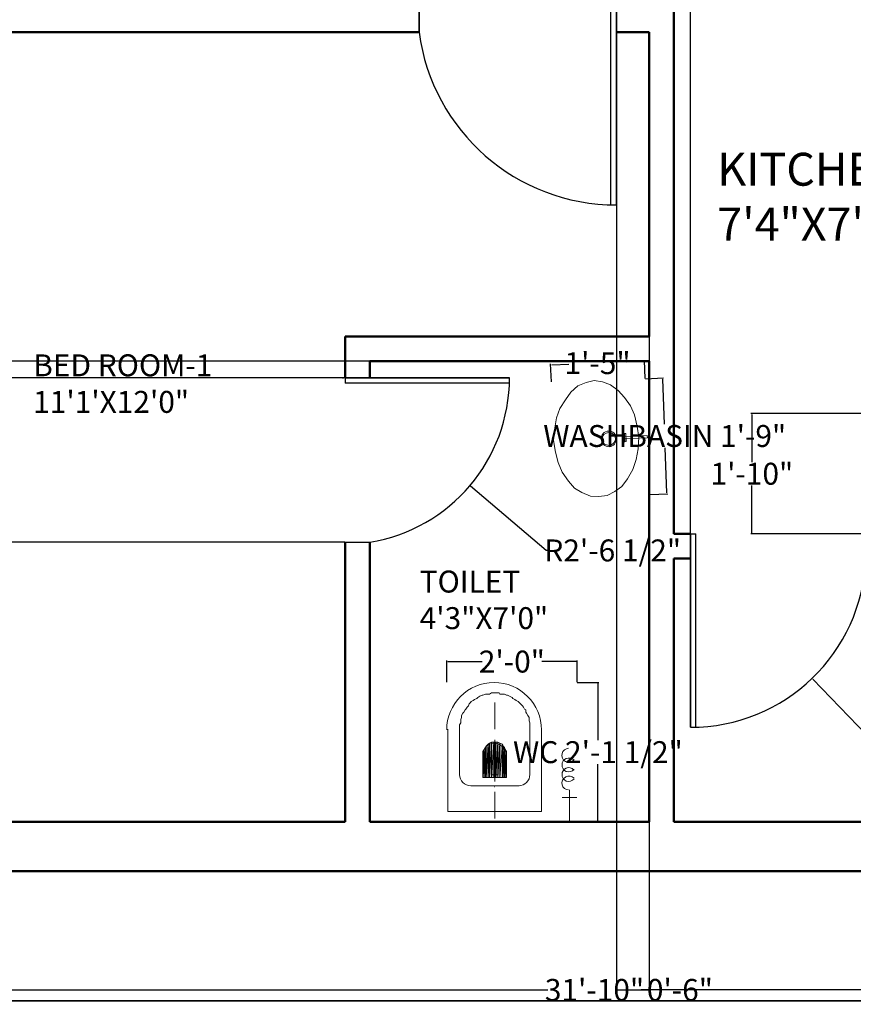
# Model space of a CAD drawing. Units: inches. Extents: x 124 to 591, y 365 to 713.
# Tile 2 of 5: x 266 to 418, y 365 to 545. Entities that reach past the tile are written whole.
import ezdxf

# ---------------------------------------------------------------- set-up
doc = ezdxf.new("R2010")
doc.units = ezdxf.units.IN
doc.header["$MEASUREMENT"] = 0
for name, color, linetype, lineweight in [('A-ANNO-DIMS', 2, 'Continuous', 18), ('A-ANNO-TTLB', 7, 'Continuous', 35), ('A-AREA-IDEN', 7, 'Continuous', 25), ('A-DOOR', 4, 'Continuous', 25), ('A-FLOR-FIXT', 8, 'Continuous', 18), ('A-WALL', 7, 'Continuous', 50)]:
    doc.layers.add(name, color=color, linetype=linetype, lineweight=lineweight)
doc.styles.get("Standard").update_dxf_attribs({"font": 'arial.ttf'})
doc.dimstyles.get("Standard").update_dxf_attribs({"dimtxt": 4, "dimasz": 0.18, "dimexe": 0.18, "dimexo": 0.0625, "dimgap": 0.09, "dimtad": 0, "dimtih": 1, "dimtoh": 1, "dimdec": 1, "dimzin": 0, "dimdsep": 46, "dimlunit": 3, "dimtxsty": 'Standard', "dimcen": 0.09, "dimclrd": 6, "dimclrt": 3, "dimadec": 0, "dimazin": 0, "dimtfac": 1, "dimtdec": 1, "dimtofl": 0, "dimtmove": 0, "dimatfit": 3, "dimfxl": 1, "dimtfillclr": 6, "dimtolj": 1, "dimtzin": 0, "dimarcsym": 0})

# ---------------------------------------------------------------- blocks, each defined once
blk = doc.blocks.new('WASH')
for p, q in [((268674.25, -2306.86), (268674.25, -2306.65)), ((268674.71, -2306.29), (268675.07, -2306.29)), ((268675.53, -2306.86), (268675.53, -2306.65)), ((268674.71, -2310.15), (268675.07, -2310.15))]:
    blk.add_line(p, q)
for points in [[(268665.93, -2302.29), (268666.07, -2301.01), (268666.64, -2299.72), (268667.36, -2298.58), (268668.5, -2297.72), (268669.93, -2296.79), (268671.43, -2296.22), (268673.07, -2295.86), (268674.86, -2295.65), (268676.5, -2295.86), (268678.36, -2296.22), (268679.78, -2296.79), (268681.07, -2297.72), (268682.21, -2298.58), (268683.14, -2299.72), (268683.64, -2301.01), (268683.86, -2302.29), (268683.64, -2303.58), (268683.14, -2304.79), (268682.21, -2305.94), (268681.07, -2306.86), (268679.78, -2307.72), (268678.36, -2308.29), (268676.5, -2308.65), (268674.86, -2308.86), (268673.07, -2308.65), (268671.43, -2308.29), (268669.93, -2307.72), (268668.5, -2306.86), (268667.36, -2305.94), (268666.64, -2304.79), (268666.07, -2303.58)], [(268674.14, -2306.65), (268674.14, -2306.65)], [(268674.86, -2306.29), (268674.86, -2306.29)], [(268675.43, -2306.65), (268675.43, -2306.65)]]:
    blk.add_lwpolyline(points, close=True)
for points in [[(268674.25, -2306.65), (268675.53, -2306.65), (268675.53, -2306.65)], [(268674.25, -2306.86), (268675.53, -2306.86), (268675.53, -2306.86)], [(268674.71, -2310.15), (268674.71, -2306.29), (268674.71, -2306.29)], [(268675.07, -2310.15), (268675.07, -2306.29), (268675.07, -2306.29)]]:
    blk.add_lwpolyline(points)
for points in [[(268673.57, -2304.22), (268673.57, -2304.86), (268674.14, -2305.36), (268674.78, -2305.36), (268674.78, -2305.36), (268675.43, -2305.36), (268676, -2304.86), (268676, -2304.22), (268676, -2304.22), (268676, -2303.51), (268675.43, -2303.01), (268674.78, -2303.01), (268674.78, -2303.01), (268674.14, -2303.01), (268673.57, -2303.51), (268673.57, -2304.22)], [(268673.78, -2304.22), (268673.78, -2304.72), (268674.21, -2305.22), (268674.78, -2305.22), (268674.78, -2305.22), (268675.36, -2305.22), (268675.78, -2304.72), (268675.78, -2304.22), (268675.78, -2304.22), (268675.78, -2303.65), (268675.36, -2303.15), (268674.78, -2303.15), (268674.78, -2303.15), (268674.21, -2303.15), (268673.78, -2303.65), (268673.78, -2304.22)]]:
    blk.add_open_spline(points, degree=3, knots=[0, 0, 0, 0, 0.0625, 0.0625, 0.0625, 0.062501, 0.125, 0.125, 0.125, 0.125001, 0.1875, 0.1875, 0.1875, 0.187501, 1, 1, 1, 1])
blk = doc.blocks.new('I')
h = blk.add_hatch(color=256)
h.paths.add_polyline_path([(268653.64, -2262.22), (268658.43, -2262.22), (268653.64, -2262.01)])
h.paths.add_polyline_path([(268658.43, -2262.22), (268653.64, -2262.01), (268658.07, -2262.01)])
h.paths.add_polyline_path([(268653.64, -2262.01), (268658.07, -2262.01), (268657.71, -2262.01)])
h = blk.add_hatch(color=256)
h.paths.add_polyline_path([(268653.64, -2262.44), (268658.78, -2262.44), (268653.64, -2262.22)])
h.paths.add_polyline_path([(268658.78, -2262.44), (268653.64, -2262.22), (268658.43, -2262.22)])
h = blk.add_hatch(color=256)
h.paths.add_polyline_path([(268653.64, -2262.58), (268659, -2262.58), (268653.64, -2262.44)])
h.paths.add_polyline_path([(268659, -2262.58), (268653.64, -2262.44), (268658.78, -2262.44)])
h = blk.add_hatch(color=256)
h.paths.add_polyline_path([(268653.64, -2262.94), (268659.36, -2262.94), (268653.64, -2262.58)])
h.paths.add_polyline_path([(268659.36, -2262.94), (268653.64, -2262.58), (268659, -2262.58)])
h = blk.add_hatch(color=256)
h.paths.add_polyline_path([(268653.64, -2263.15), (268659.5, -2263.15), (268653.64, -2262.94)])
h.paths.add_polyline_path([(268659.5, -2263.15), (268653.64, -2262.94), (268659.36, -2262.94)])
h = blk.add_hatch(color=256)
h.paths.add_polyline_path([(268653.64, -2263.51), (268659.71, -2263.51), (268653.64, -2263.15)])
h.paths.add_polyline_path([(268659.71, -2263.51), (268653.64, -2263.15), (268659.5, -2263.15)])
h = blk.add_hatch(color=256)
h.paths.add_polyline_path([(268653.64, -2263.86), (268659.71, -2263.86), (268653.64, -2263.51)])
h.paths.add_polyline_path([(268659.71, -2263.86), (268653.64, -2263.51), (268659.71, -2263.51)])
h = blk.add_hatch(color=256)
h.paths.add_polyline_path([(268653.64, -2264.22), (268659.71, -2264.22), (268653.64, -2263.86)])
h.paths.add_polyline_path([(268659.71, -2264.22), (268653.64, -2263.86), (268659.71, -2263.86)])
h = blk.add_hatch(color=256)
h.paths.add_polyline_path([(268653.64, -2264.58), (268659.71, -2264.58), (268653.64, -2264.22)])
h.paths.add_polyline_path([(268659.71, -2264.58), (268653.64, -2264.22), (268659.71, -2264.22)])
h = blk.add_hatch(color=256)
h.paths.add_polyline_path([(268653.64, -2264.94), (268659.5, -2264.94), (268653.64, -2264.58)])
h.paths.add_polyline_path([(268659.5, -2264.94), (268653.64, -2264.58), (268659.71, -2264.58)])
h = blk.add_hatch(color=256)
h.paths.add_polyline_path([(268653.64, -2265.36), (268659.36, -2265.36), (268653.64, -2264.94)])
h.paths.add_polyline_path([(268659.36, -2265.36), (268653.64, -2264.94), (268659.5, -2264.94)])
h = blk.add_hatch(color=256)
h.paths.add_polyline_path([(268653.64, -2265.51), (268659, -2265.51), (268653.64, -2265.36)])
h.paths.add_polyline_path([(268659, -2265.51), (268653.64, -2265.36), (268659.36, -2265.36)])
h = blk.add_hatch(color=256)
h.paths.add_polyline_path([(268653.64, -2265.72), (268658.78, -2265.72), (268653.64, -2265.51)])
h.paths.add_polyline_path([(268658.78, -2265.72), (268653.64, -2265.51), (268659, -2265.51)])
h = blk.add_hatch(color=256)
h.paths.add_polyline_path([(268653.64, -2265.86), (268658.43, -2265.86), (268653.64, -2265.72)])
h.paths.add_polyline_path([(268658.43, -2265.86), (268653.64, -2265.72), (268658.78, -2265.72)])
h = blk.add_hatch(color=256)
h.paths.add_polyline_path([(268653.64, -2266.08), (268658.07, -2266.08), (268653.64, -2265.86)])
h.paths.add_polyline_path([(268658.07, -2266.08), (268653.64, -2265.86), (268658.43, -2265.86)])
for points in [[(268647.78, -2256.01), (268647.78, -2272.08), (268647.78, -2272.08)], [(268647.78, -2256.01), (268661.93, -2256.01), (268661.93, -2256.01)], [(268654.21, -2258.01), (268661, -2258.01), (268661, -2258.01)], [(268661, -2258.01), (268661.71, -2258.01), (268662.28, -2258.01), (268662.64, -2258.01), (268663, -2258.22), (268663.36, -2258.22), (268663.57, -2258.22), (268663.93, -2258.36), (268664.28, -2258.36), (268664.64, -2258.58), (268664.86, -2258.72), (268665.21, -2258.94), (268665.36, -2259.08), (268665.71, -2259.29), (268665.93, -2259.51), (268666.28, -2259.65), (268666.5, -2259.86), (268666.64, -2260.01), (268666.86, -2260.36), (268667, -2260.58), (268667.21, -2260.94), (268667.36, -2261.15), (268667.57, -2261.51), (268667.78, -2261.86), (268667.78, -2262.01), (268667.93, -2262.44), (268667.93, -2262.79), (268667.93, -2263.15), (268668.14, -2263.51), (268668.14, -2264.08), (268668.14, -2264.79), (268667.93, -2264.94), (268667.93, -2265.36), (268667.93, -2265.72), (268667.78, -2266.08), (268667.78, -2266.22), (268667.57, -2266.58), (268667.36, -2267.01), (268667.21, -2267.15), (268667, -2267.51), (268666.86, -2267.72), (268666.64, -2268.08), (268666.5, -2268.22), (268666.28, -2268.44), (268665.93, -2268.79), (268665.71, -2269.01), (268665.36, -2269.15), (268665.21, -2269.36), (268664.86, -2269.36), (268664.64, -2269.51), (268664.28, -2269.72), (268663.93, -2269.94), (268663.57, -2269.94), (268663.36, -2269.94), (268663, -2270.08), (268662.64, -2270.08), (268662.28, -2270.08), (268661.71, -2270.08), (268661, -2270.08)], [(268652.21, -2260.01), (268652.21, -2268.22), (268652.21, -2268.22)], [(268653.64, -2262.01), (268653.64, -2266.08), (268653.64, -2266.08)], [(268653.64, -2262.01), (268657.71, -2262.01), (268657.71, -2262.01)], [(268652, -2264.08), (268652, -2264.01), (268652, -2264.01)], [(268646.57, -2264.08), (268651.14, -2264.08), (268651.14, -2264.08)], [(268652.93, -2264.08), (268660.07, -2264.08), (268660.07, -2264.08)], [(268661.93, -2264.08), (268666.5, -2264.08), (268666.5, -2264.08)], [(268653.64, -2266.08), (268657.71, -2266.08), (268657.71, -2266.08)], [(268654.21, -2270.08), (268661, -2270.08), (268661, -2270.08)], [(268647.78, -2272.08), (268661.93, -2272.08), (268661.93, -2272.08)], [(268650.21, -2275.6), (268650.21, -2278.17), (268650.21, -2278.17)], [(268646, -2276.89), (268651.5, -2276.89), (268651.5, -2276.89)]]:
    blk.add_lwpolyline(points)
at = {"lineweight": -2}
for points in [[(268653.64, -2262.22), (268658.43, -2262.22), (268653.64, -2262.01)], [(268658.43, -2262.22), (268653.64, -2262.01), (268658.07, -2262.01)], [(268653.64, -2262.01), (268658.07, -2262.01), (268657.71, -2262.01)], [(268658.07, -2262.01), (268653.64, -2262.01), (268653.64, -2262.01)], [(268653.64, -2262.44), (268658.78, -2262.44), (268653.64, -2262.22)], [(268658.78, -2262.44), (268653.64, -2262.22), (268658.43, -2262.22)], [(268653.64, -2262.58), (268659, -2262.58), (268653.64, -2262.44)], [(268659, -2262.58), (268653.64, -2262.44), (268658.78, -2262.44)], [(268653.64, -2262.94), (268659.36, -2262.94), (268653.64, -2262.58)], [(268659.36, -2262.94), (268653.64, -2262.58), (268659, -2262.58)], [(268653.64, -2263.15), (268659.5, -2263.15), (268653.64, -2262.94)], [(268659.5, -2263.15), (268653.64, -2262.94), (268659.36, -2262.94)], [(268653.64, -2263.51), (268659.71, -2263.51), (268653.64, -2263.15)], [(268659.71, -2263.51), (268653.64, -2263.15), (268659.5, -2263.15)], [(268653.64, -2263.86), (268659.71, -2263.86), (268653.64, -2263.51)], [(268659.71, -2263.86), (268653.64, -2263.51), (268659.71, -2263.51)], [(268653.64, -2264.22), (268659.71, -2264.22), (268653.64, -2263.86)], [(268659.71, -2264.22), (268653.64, -2263.86), (268659.71, -2263.86)], [(268653.64, -2264.58), (268659.71, -2264.58), (268653.64, -2264.22)], [(268659.71, -2264.58), (268653.64, -2264.22), (268659.71, -2264.22)], [(268653.64, -2264.94), (268659.5, -2264.94), (268653.64, -2264.58)], [(268659.5, -2264.94), (268653.64, -2264.58), (268659.71, -2264.58)], [(268653.64, -2265.36), (268659.36, -2265.36), (268653.64, -2264.94)], [(268659.36, -2265.36), (268653.64, -2264.94), (268659.5, -2264.94)], [(268653.64, -2265.51), (268659, -2265.51), (268653.64, -2265.36)], [(268659, -2265.51), (268653.64, -2265.36), (268659.36, -2265.36)], [(268653.64, -2265.72), (268658.78, -2265.72), (268653.64, -2265.51)], [(268658.78, -2265.72), (268653.64, -2265.51), (268659, -2265.51)], [(268653.64, -2265.86), (268658.43, -2265.86), (268653.64, -2265.72)], [(268658.43, -2265.86), (268653.64, -2265.72), (268658.78, -2265.72)], [(268653.64, -2266.08), (268658.07, -2266.08), (268653.64, -2265.86)], [(268658.07, -2266.08), (268653.64, -2265.86), (268658.43, -2265.86)], [(268653.64, -2266.08), (268657.71, -2266.08)], [(268657.71, -2266.08), (268653.64, -2266.08), (268658.07, -2266.08)]]:
    blk.add_lwpolyline(points, close=True, dxfattribs=at)
for points in [[(268654.07, -2263.65), (268654, -2263.65), (268654, -2263.65)], [(268654.07, -2264.08), (268654, -2264.01), (268654, -2264.01)], [(268654.07, -2263.65), (268654.07, -2263.86), (268654.07, -2264.08)], [(268654.07, -2264.44), (268654, -2264.44), (268654, -2264.44)], [(268654.07, -2264.08), (268654.07, -2264.22), (268654.07, -2264.44)]]:
    blk.add_lwpolyline(points, dxfattribs=at)
for points, knots in [([(268661.78, -2272.08), (268666.28, -2272.08), (268669.93, -2268.44), (268669.93, -2263.94), (268669.93, -2263.94), (268669.93, -2259.44), (268666.28, -2255.79), (268661.78, -2255.79)], [0, 0, 0, 0, 0.125, 0.125, 0.125, 0.125001, 1, 1, 1, 1]), ([(268657.57, -2265.86), (268658.64, -2265.86), (268659.5, -2265.01), (268659.5, -2263.94), (268659.5, -2263.94), (268659.5, -2262.86), (268658.64, -2262.01), (268657.57, -2262.01)], [0, 0, 0, 0, 0.125, 0.125, 0.125, 0.125001, 1, 1, 1, 1]), ([(268653.5, -2277.67), (268653.86, -2277.31), (268654, -2276.67), (268653.71, -2276.24), (268653.71, -2276.24), (268653.43, -2275.74), (268652.93, -2275.46), (268652.36, -2275.6), (268652.36, -2275.6), (268651.86, -2275.74), (268651.5, -2276.24), (268651.5, -2276.74)], [0, 0, 0, 0, 0.083333, 0.083333, 0.083333, 0.083334, 0.166667, 0.166667, 0.166667, 0.166668, 1, 1, 1, 1]), ([(268654.93, -2277.6), (268655.28, -2277.31), (268655.43, -2276.74), (268655.21, -2276.31), (268655.21, -2276.31), (268655.07, -2275.89), (268654.57, -2275.6), (268654.14, -2275.6), (268654.14, -2275.6), (268653.64, -2275.6), (268653.21, -2275.89), (268653, -2276.31), (268653, -2276.31), (268652.86, -2276.81), (268653, -2277.31), (268653.36, -2277.67)], [0, 0, 0, 0, 0.0625, 0.0625, 0.0625, 0.062501, 0.125, 0.125, 0.125, 0.125001, 0.1875, 0.1875, 0.1875, 0.187501, 1, 1, 1, 1]), ([(268656.57, -2277.67), (268656.93, -2277.31), (268657.07, -2276.81), (268656.86, -2276.31), (268656.86, -2276.31), (268656.71, -2275.89), (268656.28, -2275.6), (268655.78, -2275.6), (268655.78, -2275.6), (268655.28, -2275.6), (268654.86, -2275.89), (268654.64, -2276.31), (268654.64, -2276.31), (268654.5, -2276.81), (268654.64, -2277.31), (268655, -2277.67)], [0, 0, 0, 0, 0.0625, 0.0625, 0.0625, 0.062501, 0.125, 0.125, 0.125, 0.125001, 0.1875, 0.1875, 0.1875, 0.187501, 1, 1, 1, 1]), ([(268658.64, -2276.74), (268658.64, -2276.24), (268658.21, -2275.74), (268657.71, -2275.6), (268657.71, -2275.6), (268657.21, -2275.46), (268656.64, -2275.74), (268656.36, -2276.17), (268656.36, -2276.17), (268656.14, -2276.67), (268656.21, -2277.24), (268656.57, -2277.6)], [0, 0, 0, 0, 0.083333, 0.083333, 0.083333, 0.083334, 0.166667, 0.166667, 0.166667, 0.166668, 1, 1, 1, 1])]:
    blk.add_open_spline(points, degree=3, knots=knots)
for points in [[(268654.14, -2258.01), (268653.07, -2258.01), (268652.21, -2258.86), (268652.21, -2259.94)], [(268652.21, -2268.15), (268652.21, -2269.22), (268653.07, -2270.08), (268654.14, -2270.08)]]:
    blk.add_open_spline(points, degree=3)
blk = doc.blocks.new('*D25')
at = {"layer": 'A-ANNO-DIMS', "color": 0, "lineweight": -2, "transparency": 16777216}
for p, q in [((339.14, 542.65), (339.14, 549.94)), ((339.32, 549.76), (355.21, 549.76)), ((374.96, 549.76), (359.07, 549.76)), ((375.14, 542.65), (375.14, 549.94))]:
    blk.add_line(p, q, dxfattribs=at)
at = {"layer": 'A-ANNO-DIMS', "color": 0, "transparency": 16777216}
for points in [[(339.32, 549.79), (339.32, 549.73), (339.14, 549.76)], [(374.96, 549.79), (374.96, 549.73), (375.14, 549.76)]]:
    blk.add_solid(points, dxfattribs=at)
at = {"layer": 'Defpoints', "color": 0, "transparency": 16777216}
for p in [(375.14, 549.76), (339.14, 542.59), (375.14, 542.59)]:
    blk.add_point(p, dxfattribs=at)
at = {"layer": 'A-ANNO-DIMS', "color": 0, "transparency": 16777216, "insert": (357.14, 549.76), "char_height": 4, "attachment_point": 5}
blk.add_mtext("\\A1;3'", dxfattribs=at)
blk = doc.blocks.new('DOOR-SWING-36IN')
for p, q in [((36, 36), (31.5, 36)), ((0, 1), (36, 1)), ((36, 0), (36, 1)), ((36, 0), (0, 0)), ((0, 0), (36, 0))]:
    blk.add_line(p, q)
blk.add_arc((36.32, 0), 36.32, 97.6281, 180)
blk = doc.blocks.new('*D32')
at = {"layer": 'A-ANNO-DIMS', "color": 0, "lineweight": -2, "transparency": 16777216}
for p, q in [((380.43, 479.41), (383.72, 479.54)), ((381.25, 458.27), (384.54, 458.4))]:
    blk.add_line(p, q, dxfattribs=at)
at = {"layer": 'A-ANNO-DIMS', "color": 6, "lineweight": -2, "transparency": 16777216}
for p, q in [((383.55, 479.35), (383.87, 471.12)), ((384.35, 458.57), (384.03, 466.8))]:
    blk.add_line(p, q, dxfattribs=at)
at = {"layer": 'A-ANNO-DIMS', "color": 6, "transparency": 16777216}
for points in [[(383.58, 479.35), (383.52, 479.35), (383.54, 479.53)], [(384.38, 458.57), (384.32, 458.57), (384.36, 458.39)]]:
    blk.add_solid(points, dxfattribs=at)
at = {"layer": 'Defpoints', "color": 0, "transparency": 16777216}
for p in [(383.54, 479.53), (380.37, 479.41), (381.19, 458.27)]:
    blk.add_point(p, dxfattribs=at)
at = {"layer": 'A-ANNO-DIMS', "color": 3, "transparency": 16777216, "insert": (383.95, 468.96), "char_height": 4, "attachment_point": 5}
blk.add_mtext('\\A1;WASHBASIN 1\'-9"', dxfattribs=at)
blk = doc.blocks.new('*D33')
at = {"layer": 'A-ANNO-DIMS', "color": 0, "lineweight": -2, "transparency": 16777216}
for p, q in [((363.27, 478.81), (363.14, 482.1)), ((380.37, 479.47), (380.24, 482.76))]:
    blk.add_line(p, q, dxfattribs=at)
at = {"layer": 'A-ANNO-DIMS', "color": 6, "lineweight": -2, "transparency": 16777216}
for p, q in [((363.33, 481.92), (366.48, 482.05)), ((380.07, 482.57), (376.92, 482.45))]:
    blk.add_line(p, q, dxfattribs=at)
at = {"layer": 'A-ANNO-DIMS', "color": 6, "transparency": 16777216}
for points in [[(363.33, 481.95), (363.33, 481.89), (363.15, 481.92)], [(380.07, 482.6), (380.07, 482.54), (380.25, 482.58)]]:
    blk.add_solid(points, dxfattribs=at)
at = {"layer": 'Defpoints', "color": 0, "transparency": 16777216}
for p in [(363.15, 481.92), (363.27, 478.75), (380.37, 479.41)]:
    blk.add_point(p, dxfattribs=at)
at = {"layer": 'A-ANNO-DIMS', "color": 3, "transparency": 16777216, "insert": (371.7, 482.25), "char_height": 4, "attachment_point": 5}
blk.add_mtext('\\A1;1\'-5"', dxfattribs=at)
blk = doc.blocks.new('*D34')
at = {"layer": 'A-ANNO-DIMS', "color": 0, "lineweight": -2, "transparency": 16777216}
for p, q in [((368.01, 424), (371.94, 424)), ((368.01, 398.59), (371.94, 398.59))]:
    blk.add_line(p, q, dxfattribs=at)
at = {"layer": 'A-ANNO-DIMS', "color": 6, "lineweight": -2, "transparency": 16777216}
for p, q in [((371.76, 423.82), (371.76, 413.46)), ((371.76, 398.77), (371.76, 409.14))]:
    blk.add_line(p, q, dxfattribs=at)
at = {"layer": 'A-ANNO-DIMS', "color": 6, "transparency": 16777216}
for points in [[(371.73, 423.82), (371.79, 423.82), (371.76, 424)], [(371.73, 398.77), (371.79, 398.77), (371.76, 398.59)]]:
    blk.add_solid(points, dxfattribs=at)
at = {"layer": 'Defpoints', "color": 0, "transparency": 16777216}
for p in [(367.95, 424), (371.76, 424), (367.95, 398.59)]:
    blk.add_point(p, dxfattribs=at)
at = {"layer": 'A-ANNO-DIMS', "color": 3, "transparency": 16777216, "insert": (371.76, 411.3), "char_height": 4, "attachment_point": 5}
blk.add_mtext('\\A1;WC 2\'-1 1/2"', dxfattribs=at)
blk = doc.blocks.new('*D35')
at = {"layer": 'A-ANNO-DIMS', "color": 0, "lineweight": -2, "transparency": 16777216}
for p, q in [((344.18, 424.07), (344.18, 428)), ((367.95, 424.07), (367.95, 428))]:
    blk.add_line(p, q, dxfattribs=at)
at = {"layer": 'A-ANNO-DIMS', "color": 6, "lineweight": -2, "transparency": 16777216}
for p, q in [((344.36, 427.82), (350.63, 427.82)), ((367.77, 427.82), (361.51, 427.82))]:
    blk.add_line(p, q, dxfattribs=at)
at = {"layer": 'A-ANNO-DIMS', "color": 6, "transparency": 16777216}
for points in [[(344.36, 427.85), (344.36, 427.79), (344.18, 427.82)], [(367.77, 427.85), (367.77, 427.79), (367.95, 427.82)]]:
    blk.add_solid(points, dxfattribs=at)
at = {"layer": 'Defpoints', "color": 0, "transparency": 16777216}
for p in [(344.18, 427.82), (344.18, 424), (367.95, 424)]:
    blk.add_point(p, dxfattribs=at)
at = {"layer": 'A-ANNO-DIMS', "color": 3, "transparency": 16777216, "insert": (356.07, 427.82), "char_height": 4, "attachment_point": 5}
blk.add_mtext('\\A1;2\'-0"', dxfattribs=at)
blk = doc.blocks.new('*D44')
at = {"layer": 'A-ANNO-DIMS', "color": 0, "lineweight": -2, "transparency": 16777216}
for p, q in [((180.14, 389.53), (180.14, 367.76)), ((562.14, 389.53), (562.14, 367.76))]:
    blk.add_line(p, q, dxfattribs=at)
at = {"layer": 'A-ANNO-DIMS', "color": 6, "lineweight": -2, "transparency": 16777216}
for p, q in [((180.32, 367.94), (362.63, 367.94)), ((561.96, 367.94), (379.65, 367.94))]:
    blk.add_line(p, q, dxfattribs=at)
at = {"layer": 'A-ANNO-DIMS', "color": 6, "transparency": 16777216}
for points in [[(180.32, 367.97), (180.32, 367.91), (180.14, 367.94)], [(561.96, 367.97), (561.96, 367.91), (562.14, 367.94)]]:
    blk.add_solid(points, dxfattribs=at)
at = {"layer": 'Defpoints', "color": 0, "transparency": 16777216}
for p in [(180.14, 389.59), (562.14, 389.59), (562.14, 367.94)]:
    blk.add_point(p, dxfattribs=at)
at = {"layer": 'A-ANNO-DIMS', "color": 3, "transparency": 16777216, "insert": (371.14, 367.94), "char_height": 4, "attachment_point": 5}
blk.add_mtext('\\A1;31\'-10"', dxfattribs=at)
blk = doc.blocks.new('*D55')
at = {"layer": 'A-ANNO-DIMS', "color": 0, "lineweight": -2, "transparency": 16777216}
for p, q in [((325.58, 479.59), (158.31, 479.59)), ((325.58, 449.59), (158.31, 449.59))]:
    blk.add_line(p, q, dxfattribs=at)
at = {"layer": 'A-ANNO-DIMS', "color": 6, "lineweight": -2, "transparency": 16777216}
for p, q in [((158.49, 479.41), (158.49, 466.72)), ((158.49, 449.77), (158.49, 462.46))]:
    blk.add_line(p, q, dxfattribs=at)
at = {"layer": 'A-ANNO-DIMS', "color": 6, "transparency": 16777216}
for points in [[(158.46, 479.41), (158.52, 479.41), (158.49, 479.59)], [(158.46, 449.77), (158.52, 449.77), (158.49, 449.59)]]:
    blk.add_solid(points, dxfattribs=at)
at = {"layer": 'Defpoints', "color": 0, "transparency": 16777216}
for p in [(158.49, 479.59), (325.64, 479.59), (325.64, 449.59)]:
    blk.add_point(p, dxfattribs=at)
at = {"layer": 'A-ANNO-DIMS', "color": 3, "transparency": 16777216, "insert": (158.49, 464.59), "char_height": 4, "attachment_point": 5}
blk.add_mtext('\\A1;2\'-6"', dxfattribs=at)
blk = doc.blocks.new('*D56')
at = {"layer": 'A-ANNO-DIMS', "color": 0, "lineweight": -2, "transparency": 16777216}
for p, q in [((330.08, 482.59), (158.31, 482.59)), ((330.08, 479.59), (158.31, 479.59))]:
    blk.add_line(p, q, dxfattribs=at)
at = {"layer": 'A-ANNO-DIMS', "color": 6, "lineweight": -2, "transparency": 16777216}
for p, q in [((158.49, 482.59), (158.49, 482.77)), ((158.49, 482.77), (158.67, 482.77)), ((158.49, 479.77), (158.49, 482.41))]:
    blk.add_line(p, q, dxfattribs=at)
at = {"layer": 'A-ANNO-DIMS', "color": 6, "transparency": 16777216}
for points in [[(158.46, 482.41), (158.52, 482.41), (158.49, 482.59)], [(158.46, 479.77), (158.52, 479.77), (158.49, 479.59)]]:
    blk.add_solid(points, dxfattribs=at)
at = {"layer": 'Defpoints', "color": 0, "transparency": 16777216}
for p in [(158.49, 482.59), (330.14, 482.59), (330.14, 479.59)]:
    blk.add_point(p, dxfattribs=at)
at = {"layer": 'A-ANNO-DIMS', "color": 3, "transparency": 16777216, "insert": (164.07, 482.77), "char_height": 4, "attachment_point": 5}
blk.add_mtext('\\A1;0\'-3"', dxfattribs=at)
blk = doc.blocks.new('*D57')
at = {"layer": 'A-ANNO-DIMS', "color": 0, "lineweight": -2, "transparency": 16777216}
for p, q in [((388.64, 451.15), (388.64, 700.92)), ((420.64, 451.15), (420.64, 700.92))]:
    blk.add_line(p, q, dxfattribs=at)
at = {"layer": 'A-ANNO-DIMS', "color": 6, "lineweight": -2, "transparency": 16777216}
for p, q in [((388.82, 700.74), (399.2, 700.74)), ((420.46, 700.74), (410.08, 700.74))]:
    blk.add_line(p, q, dxfattribs=at)
at = {"layer": 'A-ANNO-DIMS', "color": 6, "transparency": 16777216}
for points in [[(388.82, 700.77), (388.82, 700.71), (388.64, 700.74)], [(420.46, 700.77), (420.46, 700.71), (420.64, 700.74)]]:
    blk.add_solid(points, dxfattribs=at)
at = {"layer": 'Defpoints', "color": 0, "transparency": 16777216}
for p in [(420.64, 700.74), (388.64, 451.09), (420.64, 451.09)]:
    blk.add_point(p, dxfattribs=at)
at = {"layer": 'A-ANNO-DIMS', "color": 3, "transparency": 16777216, "insert": (404.64, 700.74), "char_height": 4, "attachment_point": 5}
blk.add_mtext('\\A1;2\'-8"', dxfattribs=at)
blk = doc.blocks.new('*D60')
at = {"layer": 'A-ANNO-DIMS', "color": 0, "lineweight": -2, "transparency": 16777216}
for p, q in [((375.14, 542.53), (375.14, 367.76)), ((381.14, 542.53), (381.14, 367.76))]:
    blk.add_line(p, q, dxfattribs=at)
at = {"layer": 'A-ANNO-DIMS', "color": 6, "lineweight": -2, "transparency": 16777216}
for p, q in [((375.32, 367.94), (380.96, 367.94)), ((381.14, 367.94), (381.32, 367.94))]:
    blk.add_line(p, q, dxfattribs=at)
at = {"layer": 'A-ANNO-DIMS', "color": 6, "transparency": 16777216}
for points in [[(375.32, 367.97), (375.32, 367.91), (375.14, 367.94)], [(380.96, 367.97), (380.96, 367.91), (381.14, 367.94)]]:
    blk.add_solid(points, dxfattribs=at)
at = {"layer": 'Defpoints', "color": 0, "transparency": 16777216}
for p in [(375.14, 542.59), (381.14, 542.59), (381.14, 367.94)]:
    blk.add_point(p, dxfattribs=at)
at = {"layer": 'A-ANNO-DIMS', "color": 3, "transparency": 16777216, "insert": (386.72, 367.94), "char_height": 4, "attachment_point": 5}
blk.add_mtext('\\A1;0\'-6"', dxfattribs=at)
blk = doc.blocks.new('*D64')
at = {"layer": 'A-ANNO-DIMS', "color": 0, "lineweight": -2, "transparency": 16777216}
for p, q in [((421.43, 473.07), (399.67, 473.07)), ((421.43, 451.09), (399.67, 451.09))]:
    blk.add_line(p, q, dxfattribs=at)
at = {"layer": 'A-ANNO-DIMS', "color": 6, "lineweight": -2, "transparency": 16777216}
for p, q in [((399.85, 472.89), (399.85, 464.21)), ((399.85, 451.27), (399.85, 459.95))]:
    blk.add_line(p, q, dxfattribs=at)
at = {"layer": 'A-ANNO-DIMS', "color": 6, "transparency": 16777216}
for points in [[(399.82, 472.89), (399.88, 472.89), (399.85, 473.07)], [(399.82, 451.27), (399.88, 451.27), (399.85, 451.09)]]:
    blk.add_solid(points, dxfattribs=at)
at = {"layer": 'Defpoints', "color": 0, "transparency": 16777216}
for p in [(399.85, 473.07), (421.5, 473.07), (421.5, 451.09)]:
    blk.add_point(p, dxfattribs=at)
at = {"layer": 'A-ANNO-DIMS', "color": 3, "transparency": 16777216, "insert": (399.85, 462.08), "char_height": 4, "attachment_point": 5}
blk.add_mtext('\\A1;1\'-10"', dxfattribs=at)
blk = doc.blocks.new('*D69')
at = {"layer": 'A-ANNO-DIMS', "color": 0, "lineweight": -2, "transparency": 16777216}
for p, q in [((388.55, 447.85), (388.73, 447.85)), ((388.64, 447.76), (388.64, 447.94))]:
    blk.add_line(p, q, dxfattribs=at)
at = {"layer": 'A-ANNO-DIMS', "color": 6, "lineweight": -2, "transparency": 16777216}
for p, q in [((424.15, 410.91), (410.96, 424.64)), ((424.33, 410.91), (424.15, 410.91))]:
    blk.add_line(p, q, dxfattribs=at)
at = {"layer": 'A-ANNO-DIMS', "color": 6, "transparency": 16777216}
blk.add_solid([(410.98, 424.66), (410.94, 424.62), (410.83, 424.77)], dxfattribs=at)
at = {"layer": 'Defpoints', "color": 0, "transparency": 16777216}
for p in [(388.64, 447.85), (410.83, 424.77)]:
    blk.add_point(p, dxfattribs=at)
at = {"layer": 'A-ANNO-DIMS', "color": 3, "transparency": 16777216, "insert": (431.65, 410.91), "char_height": 4, "attachment_point": 5}
blk.add_mtext('\\A1;R2\'-8"', dxfattribs=at)
blk = doc.blocks.new('*D70')
at = {"layer": 'A-ANNO-DIMS', "color": 0, "lineweight": -2, "transparency": 16777216}
for p, q in [((325.15, 479.59), (325.33, 479.59)), ((325.24, 479.5), (325.24, 479.68))]:
    blk.add_line(p, q, dxfattribs=at)
at = {"layer": 'A-ANNO-DIMS', "color": 6, "lineweight": -2, "transparency": 16777216}
for p, q in [((362.3, 448.09), (348.54, 459.79)), ((362.48, 448.09), (362.3, 448.09))]:
    blk.add_line(p, q, dxfattribs=at)
at = {"layer": 'A-ANNO-DIMS', "color": 6, "transparency": 16777216}
blk.add_solid([(348.56, 459.81), (348.52, 459.77), (348.4, 459.91)], dxfattribs=at)
at = {"layer": 'Defpoints', "color": 0, "transparency": 16777216}
for p in [(325.24, 479.59), (348.4, 459.91)]:
    blk.add_point(p, dxfattribs=at)
at = {"layer": 'A-ANNO-DIMS', "color": 3, "transparency": 16777216, "insert": (374.46, 448.09), "char_height": 4, "attachment_point": 5}
blk.add_mtext('\\A1;R2\'-6 1/2"', dxfattribs=at)

msp = doc.modelspace()

# ---------------------------------------------------------------- linework, layer by layer
at = {"layer": 'A-ANNO-TTLB'}
msp.add_lwpolyline([(124.09, 712.7), (590.57, 712.7), (590.57, 365.95), (124.09, 365.95)], close=True, dxfattribs=at)
msp.add_lwpolyline([(124.09, 712.7), (590.57, 712.7), (590.57, 365.95), (124.09, 365.95)], close=True, dxfattribs=at)
at = {"layer": 'A-DOOR'}
for p, q in [((325.64, 479.59), (355.64, 479.59)), ((355.64, 479.59), (325.64, 479.59)), ((325.64, 479.59), (325.64, 478.59)), ((355.64, 478.59), (325.64, 478.59)), ((388.64, 451.09), (388.64, 415.83)), ((388.64, 415.83), (388.64, 451.09)), ((388.64, 451.09), (389.64, 451.09)), ((389.64, 415.84), (389.64, 451.09)), ((325.64, 449.59), (330.14, 449.59))]:
    msp.add_line(p, q, dxfattribs=at)
for centre, radius, start, end in [((325.24, 479.59), 30.4, 279.2709, 0), ((388.64, 447.85), 32.02, 270, 357.7413)]:
    msp.add_arc(centre, radius, start, end, dxfattribs=at)
at = {"layer": 'A-WALL'}
for p, q in [((385.64, 547.09), (385.64, 451.09)), ((189.14, 542.59), (339.14, 542.59)), ((375.14, 542.59), (381.14, 542.59)), ((381.14, 542.59), (381.14, 487.09)), ((325.64, 487.09), (325.64, 479.59)), ((325.64, 487.09), (381.14, 487.09)), ((325.64, 482.59), (325.64, 479.59)), ((330.14, 482.59), (330.14, 479.59)), ((330.14, 482.59), (381.14, 482.59)), ((381.14, 482.59), (381.14, 398.59)), ((385.64, 451.09), (388.64, 451.09)), ((385.64, 451.09), (388.64, 451.09)), ((325.64, 449.59), (325.64, 398.59)), ((330.14, 449.59), (330.14, 398.59)), ((385.64, 446.59), (388.64, 446.59)), ((385.64, 446.59), (385.64, 398.59)), ((189.14, 398.59), (325.64, 398.59)), ((330.14, 398.59), (381.14, 398.59)), ((385.64, 398.59), (472.64, 398.59)), ((180.14, 389.59), (562.14, 389.59))]:
    msp.add_line(p, q, dxfattribs=at)

# ---------------------------------------------------------------- block references
at = {"layer": 'A-DOOR', "rotation": 89.99999999999976}
msp.add_blockref('DOOR-SWING-36IN', (375.14, 511.09), dxfattribs=at)
at = {"layer": 'A-FLOR-FIXT'}
for name, p, xscale, yscale, zscale, rotation in [('WASH', (9886.28, -316436.73), 1.179999999999999, 1.179999999999999, 1.179999999999999, 92.21069281596569), ('I', (-2051.47, -284903.46), 1.061999999999999, 1.061999999999999, 1.061999999999999, 89.99999999997907)]:
    msp.add_blockref(name, p, dxfattribs=dict(at, xscale=xscale, yscale=yscale, zscale=zscale, rotation=rotation))

# ---------------------------------------------------------------- texts
at = {"layer": 'A-AREA-IDEN', "attachment_point": 1}
for s, width, insert, char_height in [('KITCHEN\\P7\'4"X7\'7"', 40.647, (393.54, 520.61), 6), ('BED ROOM-1\\P11\'1\'X12\'0"', 53.483, (268.75, 483.85), 4), ('TOILET\\P4\'3"X7\'0"', 33.3568, (339.25, 444.41), 4)]:
    msp.add_mtext_dynamic_manual_height_columns(s, width=width, gutter_width=1, heights=[0], dxfattribs=dict(at, insert=insert, char_height=char_height))

# ---------------------------------------------------------------- dimensions: what is measured, and where the dimension line sits
at = {"layer": 'A-ANNO-DIMS'}
for base, p1, p2, override, picture, middle in [((420.64, 700.74), (388.64, 451.09), (420.64, 451.09), {"dimdec": 1, "dimlfac": 1, "dimrnd": 0, "dimzin": 1, "dimdsep": 46, "dimlunit": 4, "dimfrac": 2}, '*D57', (404.64, 700.74)), ((375.14, 549.76), (339.14, 542.59), (375.14, 542.59), {"dimclrd": 0, "dimclre": 0, "dimclrt": 0}, '*D25', (357.14, 549.76)), ((381.14, 367.94), (375.14, 542.59), (381.14, 542.59), {"dimdec": 1, "dimlfac": 1, "dimrnd": 0, "dimzin": 1, "dimdsep": 46, "dimlunit": 4, "dimfrac": 2}, '*D60', (386.72, 367.94)), ((562.14, 367.94), (180.14, 389.59), (562.14, 389.59), {"dimdec": 1, "dimlfac": 1, "dimrnd": 0, "dimzin": 1, "dimdsep": 46, "dimlunit": 4, "dimfrac": 2}, '*D44', (371.14, 367.94))]:
    dim = msp.add_linear_dim(base=base, p1=p1, p2=p2, dimstyle='Standard', override=override, dxfattribs=at)
    dim.commit()
    dim.dimension.update_dxf_attribs({"geometry": picture, "text_midpoint": middle})
for base, p1, p2, angle, picture, middle in [((158.49, 482.59), (330.14, 479.59), (330.14, 482.59), 90, '*D56', (164.07, 482.77)), ((363.15, 481.92), (380.37, 479.41), (363.27, 478.75), 182.2107, '*D33', (371.7, 482.25)), ((158.49, 479.59), (325.64, 449.59), (325.64, 479.59), 90, '*D55', (158.49, 464.59)), ((399.85, 473.07), (421.5, 451.09), (421.5, 473.07), 90, '*D64', (399.85, 462.08)), ((344.18, 427.82), (367.95, 424), (344.18, 424), 180, '*D35', (356.07, 427.82))]:
    dim = msp.add_linear_dim(base=base, p1=p1, p2=p2, angle=angle, dimstyle='Standard', override={"dimdec": 1, "dimlfac": 1, "dimrnd": 0, "dimzin": 1, "dimdsep": 46, "dimlunit": 4, "dimfrac": 2}, dxfattribs=at)
    dim.commit()
    dim.dimension.update_dxf_attribs({"geometry": picture, "text_midpoint": middle})
for center, mpoint, picture, middle in [((325.24, 479.59), (348.4, 459.91), '*D70', (374.46, 448.09)), ((388.64, 447.85), (410.83, 424.77), '*D69', (431.65, 410.91))]:
    dim = msp.add_radius_dim(center=center, mpoint=mpoint, dimstyle='Standard', override={"dimdec": 1, "dimlfac": 1, "dimrnd": 0, "dimzin": 1, "dimdsep": 46, "dimlunit": 4, "dimfrac": 2}, dxfattribs=at)
    dim.commit()
    dim.dimension.update_dxf_attribs({"geometry": picture, "text_midpoint": middle, "dimtype": 164})
for base, p1, p2, angle, text, picture, middle in [((383.54, 479.53), (381.19, 458.27), (380.37, 479.41), 92.2107, 'WASHBASIN <>', '*D32', (383.95, 468.96)), ((371.76, 424), (367.95, 398.59), (367.95, 424), 90, 'WC <>', '*D34', (371.76, 411.3))]:
    dim = msp.add_linear_dim(base=base, p1=p1, p2=p2, angle=angle, text=text, dimstyle='Standard', override={"dimdec": 1, "dimlfac": 1, "dimrnd": 0, "dimzin": 1, "dimdsep": 46, "dimlunit": 4, "dimfrac": 2}, dxfattribs=at)
    dim.commit()
    dim.dimension.update_dxf_attribs({"geometry": picture, "text_midpoint": middle})

doc.saveas('drawing.dxf')
